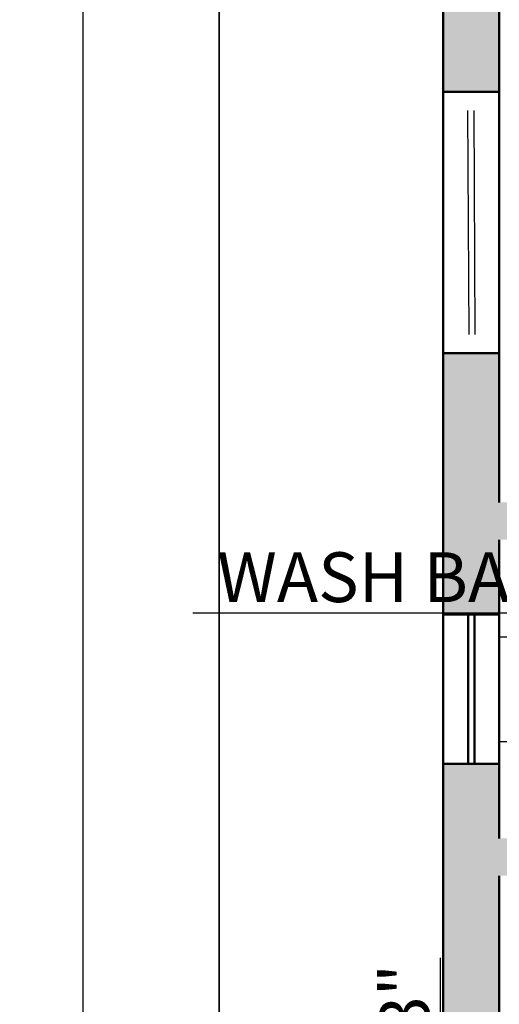
# Model space of a CAD drawing. Units: inches. Extents: x 1986 to 21484, y -1816 to 2016.
# Tile 6 of 85: x 2010 to 2087, y 1607 to 1765. Entities that reach past the tile are written whole.
import ezdxf

# ---------------------------------------------------------------- set-up
doc = ezdxf.new("R2010")
doc.units = ezdxf.units.IN
for name, color, linetype, lineweight in [('A-ANNO-DIMS', 2, 'Continuous', 18), ('A-FLOR-FIXT', 8, 'Continuous', 18), ('A-GLAZ', 4, 'Continuous', 25), ('A-WALL', 7, 'Continuous', 50), ('A-WALL-PATT', 8, 'Continuous', 13), ('C-PROP', 7, 'Continuous', 35)]:
    doc.layers.add(name, color=color, linetype=linetype, lineweight=lineweight)
doc.layers.add('SANTEH', color=7, linetype='Continuous')
doc.styles.get("Standard").update_dxf_attribs({"font": 'arial.ttf'})
doc.dimstyles.new('ISO-25', dxfattribs={"dimtxt": 8, "dimasz": 2.5, "dimexe": 1.25, "dimexo": 0.625, "dimtad": 1, "dimdec": 1, "dimlunit": 3, "dimtxsty": 'Standard', "dimcen": 2.5, "dimadec": 0, "dimazin": 0, "dimtfac": 1, "dimtdec": 1, "dimtmove": 0, "dimatfit": 3, "dimfxl": 1, "dimarcsym": 0})

# ---------------------------------------------------------------- blocks, each defined once
blk = doc.blocks.new('*D2')
at = {"layer": 'A-ANNO-DIMS', "color": 0, "lineweight": -2, "transparency": 16777216}
for p, q in [((2041.69, 1900.75), (2019.21, 1900.75)), ((2020.46, 1898.25), (2020.46, 1069.25)), ((2041.69, 1066.75), (2019.21, 1066.75))]:
    blk.add_line(p, q, dxfattribs=at)
at = {"layer": 'A-ANNO-DIMS', "color": 0, "transparency": 16777216}
for points in [[(2020.05, 1898.25), (2020.88, 1898.25), (2020.46, 1900.75)], [(2020.05, 1069.25), (2020.88, 1069.25), (2020.46, 1066.75)]]:
    blk.add_solid(points, dxfattribs=at)
at = {"layer": 'Defpoints', "color": 0, "transparency": 16777216}
for p in [(2042.31, 1900.75), (2020.46, 1066.75), (2042.31, 1066.75)]:
    blk.add_point(p, dxfattribs=at)
at = {"layer": 'A-ANNO-DIMS', "color": 0, "transparency": 16777216, "insert": (2015.75, 1483.75), "char_height": 8, "attachment_point": 5, "rotation": 90}
blk.add_mtext('69\'-6"', dxfattribs=at)
blk = doc.blocks.new('WC 2 Symb_109')
at = {"layer": 'SANTEH'}
for p, q in [((0, 0), (0, 380)), ((0, 380), (132.4, 380)), ((153.6, 364.9), (506.8, 364.9)), ((506.3, 364.9), (215.7, 330.9)), ((506.3, 356), (215.7, 322)), ((215.7, 190), (215.7, 330.9)), ((215.7, 190), (215.7, 49.1)), ((506.3, 24), (215.7, 58)), ((506.3, 15.1), (215.7, 49.1)), ((153.8, 15.1), (506.8, 15.1)), ((0, 0), (132.4, 0))]:
    blk.add_line(p, q, dxfattribs=at)
for points in [[(154.6, 360.1), (153.9, 364.1), (152.3, 367.9), (150.2, 371.3), (147.4, 374.3), (144.1, 376.7), (140.5, 378.5), (136.5, 379.6), (132.4, 380)], [(154.6, 19.7), (158.6, 62.1), (161.4, 104.7), (163.1, 147.3), (163.7, 189.9), (163.1, 232.5), (161.4, 275.1), (158.6, 317.7), (154.6, 360.1)], [(506.8, 15.1), (569.2, 28.4), (622.2, 66.3), (657.6, 123.1), (670, 190), (657.6, 256.9), (622.2, 313.7), (569.2, 351.6), (506.8, 364.9)], [(506.3, 24), (565.5, 36.6), (615.7, 72.6), (649.2, 126.5), (661, 190), (649.2, 253.5), (615.7, 307.4), (565.5, 343.4), (506.3, 356)], [(132.4, 0), (136.5, 0.4), (140.4, 1.5), (144.1, 3.2), (147.3, 5.6), (150.1, 8.6), (152.3, 12), (153.8, 15.7), (154.6, 19.7)]]:
    blk.add_lwpolyline(points, dxfattribs=at)
blk.add_lwpolyline([(83.6, 208.5), (70.4, 203.1), (64.9, 190), (70.4, 176.9), (83.6, 171.5), (96.8, 176.9), (102.2, 190), (96.8, 203.1)], close=True, dxfattribs=at)
blk = doc.blocks.new('WIN-36')
for p, q in [((0, 36), (0, 0)), ((0, 36), (0, 0)), ((1, 36), (1, 0))]:
    blk.add_line(p, q)
blk = doc.blocks.new('*D101')
at = {"layer": 'A-ANNO-DIMS', "color": 0, "lineweight": -2, "transparency": 16777216}
for p, q in [((2164.21, 1671.28), (2164.21, 1668.69)), ((2177.31, 1671.28), (2177.31, 1668.69)), ((2164.21, 1669.94), (2038.09, 1669.94)), ((2174.81, 1669.94), (2166.71, 1669.94))]:
    blk.add_line(p, q, dxfattribs=at)
at = {"layer": 'A-ANNO-DIMS', "color": 0, "transparency": 16777216}
for points in [[(2166.71, 1670.35), (2166.71, 1669.52), (2164.21, 1669.94)], [(2174.81, 1670.35), (2174.81, 1669.52), (2177.31, 1669.94)]]:
    blk.add_solid(points, dxfattribs=at)
at = {"layer": 'Defpoints', "color": 0, "transparency": 16777216}
for p in [(2164.21, 1671.9), (2177.31, 1671.9), (2164.21, 1669.94)]:
    blk.add_point(p, dxfattribs=at)
at = {"layer": 'A-ANNO-DIMS', "color": 0, "transparency": 16777216, "insert": (2099.9, 1674.7), "char_height": 8, "attachment_point": 5}
blk.add_mtext('WASH BASIN 1\'-1" TYP.', dxfattribs=at)
blk = doc.blocks.new('*D119')
at = {"layer": 'A-ANNO-DIMS', "color": 0, "lineweight": -2, "transparency": 16777216}
for p, q in [((2077.86, 1542.78), (2077.86, 1614.56)), ((2086.69, 1542.78), (2076.61, 1542.78)), ((2077.86, 1482.29), (2077.86, 1540.28)), ((2086.69, 1479.79), (2076.61, 1479.79))]:
    blk.add_line(p, q, dxfattribs=at)
at = {"layer": 'A-ANNO-DIMS', "color": 0, "transparency": 16777216}
for points in [[(2077.45, 1540.28), (2078.28, 1540.28), (2077.86, 1542.78)], [(2077.45, 1482.29), (2078.28, 1482.29), (2077.86, 1479.79)]]:
    blk.add_solid(points, dxfattribs=at)
at = {"layer": 'Defpoints', "color": 0, "transparency": 16777216}
for p in [(2077.86, 1542.78), (2087.31, 1542.78), (2087.31, 1479.79)]:
    blk.add_point(p, dxfattribs=at)
at = {"layer": 'A-ANNO-DIMS', "color": 0, "transparency": 16777216, "insert": (2073.15, 1579.92), "char_height": 8, "attachment_point": 5, "rotation": 90}
blk.add_mtext('TV UNIT 5\'-3"', dxfattribs=at)

msp = doc.modelspace()

# ---------------------------------------------------------------- hatches: boundary and pattern name
at = {"layer": 'A-WALL-PATT'}
h = msp.add_hatch(color=256, dxfattribs=at)
h.dxf.hatch_style = 1
h.paths.add_polyline_path([(2087.31, 1843.75), (2135.31, 1843.75), (2135.31, 1852.75), (2078.31, 1852.75), (2078.31, 1753.75), (2087.31, 1753.75)])
h.paths.add_polyline_path([(2231.31, 1852.75), (2177.31, 1852.75), (2177.31, 1843.75), (2225.31, 1843.75), (2225.31, 1627.75), (2231.31, 1627.75), (2231.31, 1633.35), (2231.31, 1676.45), (2231.31, 1678.13)])
h.paths.add_polyline_path([(2384.31, 1852.75), (2261.31, 1852.75), (2261.31, 1843.75), (2375.31, 1843.75), (2375.31, 1795.75), (2279.31, 1795.75), (2279.31, 1813.75), (2273.31, 1813.75), (2273.31, 1789.75), (2375.31, 1789.75), (2375.31, 1741.75), (2384.31, 1741.75)])
h.paths.add_polyline_path([(2384.31, 1705.75), (2375.31, 1705.75), (2375.31, 1600.75), (2384.31, 1600.75)])
h.paths.add_polyline_path([(2384.31, 1564.75), (2375.31, 1564.75), (2375.31, 1537.75), (2293.31, 1537.75), (2293.31, 1531.75), (2375.31, 1531.75), (2384.31, 1531.75)])
h.paths.add_polyline_path([(2087.31, 1711.75), (2078.31, 1711.75), (2078.31, 1669.75), (2087.31, 1669.75), (2087.31, 1681.75), (2177.31, 1681.75), (2177.31, 1663.75), (2183.31, 1663.75), (2183.31, 1681.75), (2189.31, 1681.75), (2189.31, 1687.75), (2087.31, 1687.75)])
h.paths.add_polyline_path([(2087.31, 1627.75), (2183.31, 1627.75), (2183.31, 1633.75), (2153.31, 1633.75), (2087.31, 1633.75), (2087.31, 1645.75), (2078.31, 1645.75), (2078.31, 1441.75), (2087.31, 1441.75)])
h.paths.add_polyline_path([(2087.31, 1399.75), (2078.31, 1399.75), (2078.31, 1276.75), (2087.31, 1276.75)])
h.paths.add_polyline_path([(2151.81, 1387.75), (2135.31, 1387.75), (2135.31, 1378.75), (2151.81, 1378.75)])
h.paths.add_polyline_path([(2219.31, 1387.75), (2193.81, 1387.75), (2193.81, 1378.75), (2210.31, 1378.75), (2210.31, 1189.75), (2219.31, 1189.75)])
h.paths.add_polyline_path([(2384.31, 1387.75), (2375.31, 1387.75), (2255.31, 1387.75), (2255.31, 1381.75), (2375.31, 1381.75), (2375.31, 1363.75), (2384.31, 1363.75)])
h.paths.add_polyline_path([(2384.31, 1339.75), (2375.31, 1339.75), (2375.31, 1321.75), (2279.31, 1321.75), (2279.31, 1351.75), (2273.31, 1351.75), (2273.31, 1315.75), (2375.31, 1315.75), (2375.31, 1303.75), (2384.31, 1303.75)])
h.paths.add_polyline_path([(2225.31, 1123.75), (2219.31, 1123.75), (2219.31, 1147.75), (2210.31, 1147.75), (2210.31, 1114.75), (2225.31, 1114.75)])
h.paths.add_polyline_path([(2384.31, 1147.75), (2375.31, 1147.75), (2375.31, 1123.75), (2267.31, 1123.75), (2267.31, 1114.75), (2384.31, 1114.75)])
h.paths.add_polyline_path([(2384.31, 1261.75), (2375.31, 1261.75), (2375.31, 1189.75), (2384.31, 1189.75)])
h.paths.add_polyline_path([(2384.31, 1441.75), (2375.31, 1441.75), (2375.31, 1423.75), (2384.31, 1423.75)])
h.paths.add_polyline_path([(2384.31, 1495.75), (2375.31, 1495.75), (2375.31, 1477.75), (2384.31, 1477.75)])

# ---------------------------------------------------------------- linework, layer by layer
at = {"layer": 'A-WALL'}
for p, q in [((2078.31, 1276.75), (2078.31, 1852.75)), ((2087.31, 1687.75), (2087.31, 1843.75)), ((2078.31, 1753.75), (2087.31, 1753.75)), ((2078.31, 1711.75), (2087.31, 1711.75)), ((2087.31, 1633.75), (2087.31, 1681.75)), ((2078.31, 1669.75), (2087.31, 1669.75)), ((2082.31, 1645.75), (2082.31, 1669.75)), ((2083.31, 1645.75), (2083.31, 1669.75)), ((2078.31, 1645.75), (2087.31, 1645.75)), ((2087.31, 1276.75), (2087.31, 1627.75))]:
    msp.add_line(p, q, dxfattribs=at)
at = {"layer": 'C-PROP'}
msp.add_lwpolyline([(2042.31, 1900.75), (2402.31, 1900.75), (2402.31, 1066.75), (2042.31, 1066.75)], close=True, dxfattribs=at)

# ---------------------------------------------------------------- block references
at = {"layer": 'A-FLOR-FIXT', "xscale": -0.0441898926459964, "yscale": 0.0441898926459964, "zscale": 0.0441898926459964, "rotation": 180}
msp.add_blockref('WC 2 Symb_109', (2087.31, 1666.15), dxfattribs=at)
at = {"layer": 'A-GLAZ', "rotation": 0.302793432207276}
msp.add_blockref('WIN-36', (2082.41, 1714.75), dxfattribs=at)

# ---------------------------------------------------------------- dimensions: what is measured, and where the dimension line sits
at = {"layer": 'A-ANNO-DIMS'}
dim = msp.add_linear_dim(base=(2020.46, 1066.75), p1=(2042.31, 1900.75), p2=(2042.31, 1066.75), angle=90, dimstyle='ISO-25', override={"dimclrd": 0, "dimclre": 0, "dimclrt": 0}, dxfattribs=at)
dim.commit()
dim.dimension.update_dxf_attribs({"geometry": '*D2', "text_midpoint": (2015.75, 1483.75)})
for base, p1, p2, angle, text, picture, middle in [((2164.21, 1669.94), (2177.31, 1671.9), (2164.21, 1671.9), 180, 'WASH BASIN <> TYP.', '*D101', (2099.9, 1674.7)), ((2077.86, 1542.78), (2087.31, 1479.79), (2087.31, 1542.78), 90, 'TV UNIT <>', '*D119', (2073.15, 1579.92))]:
    dim = msp.add_linear_dim(base=base, p1=p1, p2=p2, angle=angle, text=text, dimstyle='ISO-25', override={"dimdec": 1, "dimrnd": 0, "dimzin": 1, "dimlunit": 4, "dimfrac": 2}, dxfattribs=at)
    dim.commit()
    dim.dimension.update_dxf_attribs({"geometry": picture, "text_midpoint": middle})

doc.saveas('drawing.dxf')
